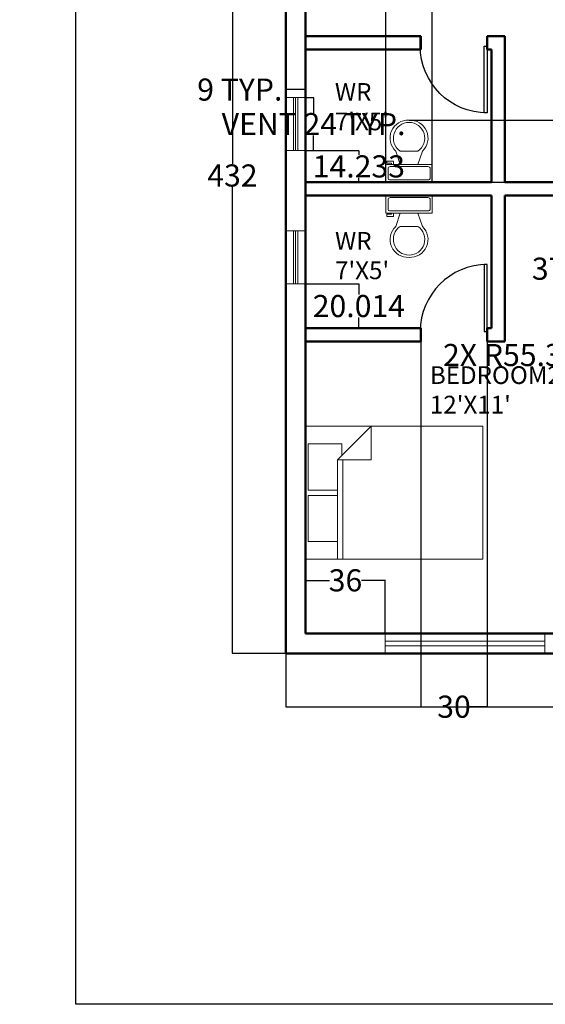
# Model space of a CAD drawing. Units: inches. Extents: x -16 to 1298, y 3 to 744.
# Tile 1 of 5: x -16 to 221, y 3 to 448. Entities that reach past the tile are written whole.
import ezdxf

# ---------------------------------------------------------------- set-up
doc = ezdxf.new("R2010")
doc.units = ezdxf.units.IN
doc.header["$MEASUREMENT"] = 0
for name, color, linetype, lineweight in [('A-ANNO-DIMS', 2, 'Continuous', 18), ('A-AREA-IDEN', 7, 'Continuous', 18), ('A-DOOR', 3, 'Continuous', 25), ('A-FLOR-FIXT', 9, 'Continuous', 18), ('A-FURN', 8, 'Continuous', 18), ('A-GLAZ', 4, 'Continuous', 18), ('A-WALL', 7, 'Continuous', 50)]:
    doc.layers.add(name, color=color, linetype=linetype, lineweight=lineweight)
doc.styles.get("Standard").update_dxf_attribs({"font": 'arial.ttf'})
doc.dimstyles.get("Standard").update_dxf_attribs({"dimtxt": 10, "dimasz": 0.18, "dimexe": 0.18, "dimexo": 0.0625, "dimgap": 0.09, "dimtad": 0, "dimtih": 1, "dimtoh": 1, "dimdec": 0, "dimzin": 0, "dimdsep": 46, "dimlunit": 3, "dimtxsty": 'Standard', "dimcen": 0.09, "dimadec": 0, "dimazin": 0, "dimtfac": 1, "dimtdec": 0, "dimtofl": 0, "dimtmove": 0, "dimatfit": 3, "dimfxl": 1, "dimtolj": 1, "dimtzin": 0, "dimarcsym": 0})

# ---------------------------------------------------------------- blocks, each defined once
blk = doc.blocks.new('Bed - Queen')
for p, q in [((0, -80.00003), (0, 0)), ((0, 0), (59.99999, 0)), ((59.99999, 0), (59.99999, -80.00003)), ((7.99999, -1.2), (28.79998, -1.2)), ((7.99999, -14.4), (7.99999, -1.2)), ((28.79998, -1.2), (28.79998, -14.4)), ((31.19999, -1.2), (51.99999, -1.2)), ((31.19999, -14.4), (31.19999, -1.2)), ((51.99999, -1.2), (51.99999, -16.4)), ((0, -14.4), (44.8, -14.4)), ((44.8, -16.8), (0, -16.8)), ((59.99999, -29.6), (44.8, -14.4)), ((44.8, -14.4), (44.8, -29.6)), ((51.99999, -16.4), (46.79936, -16.4)), ((44.8, -29.6), (59.99999, -29.6)), ((59.99999, -80.00003), (0, -80.00003))]:
    blk.add_line(p, q)
blk = doc.blocks.new('*U8')
for p, q in [((0, 0), (0, -6)), ((-40, 0), (-40, -6))]:
    blk.add_line(p, q)
blk.add_lwpolyline([(0, 0), (0, 40), (-1.75, 40), (-1.75, 0)], close=True)
blk.add_arc((0, 0), 40, 90, 180)
blk = doc.blocks.new('*U3')
for p, q in [((9.5, -6), (9.5, -2)), ((-10, -8.5), (-8, -8.5)), ((-10, -9.5), (-10, -8.5)), ((-8, -8.5), (-8, -8)), ((-7, -8), (-7, -9.5)), ((-4, -8), (-6, -14)), ((4, -8), (6, -14)), ((-7, -9.5), (-10, -9.5)), ((4, -14), (-4, -14))]:
    blk.add_line(p, q)
blk.add_lwpolyline([(10.5, -8), (10.5, 0), (-10.5, 0), (-10.5, -8)], close=True)
for points in [[(-9.5, -2), (-9.5, -6)], [(8.5, -1), (-8.5, -1)], [(-8.5, -7), (8.5, -7)]]:
    blk.add_lwpolyline(points)
for centre, radius, start, end in [((-8.625, -1.875), 0.8839, 81.8699, 188.1301), ((8.625, -1.875), 0.8839, 351.8699, 98.1301), ((-8.625, -6.125), 0.8839, 171.869898, 278.1301), ((8.625, -6.125), 0.8839, 261.8699, 8.1301), ((-0.4772, -19.9188), 8.0953, 133.01722, 273.38), ((0.0374, -19.8731), 7.127, 124.50543, 269.7), ((-0.0373, -19.8731), 7.127, 270.3, 55.4946), ((0.4773, -19.9188), 8.0953, 266.62, 46.9828)]:
    blk.add_arc(centre, radius, start, end)
blk = doc.blocks.new('WIN-72-WALL-9')
for p, q in [((0, 0), (0, 9)), ((72, 0), (72, 9)), ((72, 5.5), (0, 5.5)), ((72, 3.5), (0, 3.5))]:
    blk.add_line(p, q)
blk = doc.blocks.new('VENT-24-WALL-9')
for p, q in [((0, 0), (0, 9)), ((24, 0), (24, 9)), ((0, 5.5), (24, 5.5)), ((0, 4.5), (24, 4.5)), ((0, 3.5), (24, 3.5))]:
    blk.add_line(p, q)
blk = doc.blocks.new('*D28')
at = {"layer": 'A-ANNO-DIMS', "color": 0, "lineweight": -2, "transparency": 16777216}
for p, q in [((112.74, 413.22), (116.46, 413.22)), ((116.28, 413.04), (116.28, 406.34)), ((116.28, 389.4), (116.28, 396.11)), ((112.74, 389.22), (116.46, 389.22))]:
    blk.add_line(p, q, dxfattribs=at)
at = {"layer": 'A-ANNO-DIMS', "color": 0, "transparency": 16777216}
for points in [[(116.25, 413.04), (116.31, 413.04), (116.28, 413.22)], [(116.25, 389.4), (116.31, 389.4), (116.28, 389.22)]]:
    blk.add_solid(points, dxfattribs=at)
at = {"layer": 'Defpoints', "color": 0, "transparency": 16777216}
for p in [(112.68, 413.22), (116.28, 413.22), (112.68, 389.22)]:
    blk.add_point(p, dxfattribs=at)
at = {"layer": 'A-ANNO-DIMS', "color": 0, "transparency": 16777216, "insert": (116.28, 401.22), "char_height": 10, "attachment_point": 5}
blk.add_mtext('\\A1;VENT 24 TYP.', dxfattribs=at)
blk = doc.blocks.new('*D29')
at = {"layer": 'A-ANNO-DIMS', "color": 0, "lineweight": -2, "transparency": 16777216}
for p, q in [((103.68, 416.82), (103.5, 416.82)), ((103.68, 413.28), (103.68, 417)), ((112.5, 416.82), (103.86, 416.82)), ((112.68, 413.28), (112.68, 417))]:
    blk.add_line(p, q, dxfattribs=at)
at = {"layer": 'A-ANNO-DIMS', "color": 0, "transparency": 16777216}
for points in [[(103.86, 416.85), (103.86, 416.79), (103.68, 416.82)], [(112.5, 416.85), (112.5, 416.79), (112.68, 416.82)]]:
    blk.add_solid(points, dxfattribs=at)
at = {"layer": 'Defpoints', "color": 0, "transparency": 16777216}
for p in [(103.68, 416.82), (103.68, 413.22), (112.68, 413.22)]:
    blk.add_point(p, dxfattribs=at)
at = {"layer": 'A-ANNO-DIMS', "color": 0, "transparency": 16777216, "insert": (82.95, 416.82), "char_height": 10, "attachment_point": 5}
blk.add_mtext('\\A1;9 TYP.', dxfattribs=at)
blk = doc.blocks.new('*D30')
at = {"layer": 'A-ANNO-DIMS', "color": 0, "lineweight": -2, "transparency": 16777216}
for p, q in [((112.68, 484.49), (112.68, 472.37)), ((192.68, 484.49), (192.68, 472.37)), ((112.68, 472.55), (112.5, 472.55)), ((192.5, 472.55), (112.86, 472.55))]:
    blk.add_line(p, q, dxfattribs=at)
at = {"layer": 'A-ANNO-DIMS', "color": 0, "transparency": 16777216}
for points in [[(112.86, 472.58), (112.86, 472.52), (112.68, 472.55)], [(192.5, 472.58), (192.5, 472.52), (192.68, 472.55)]]:
    blk.add_solid(points, dxfattribs=at)
at = {"layer": 'Defpoints', "color": 0, "transparency": 16777216}
for p in [(112.68, 484.55), (192.68, 484.55), (112.68, 472.55)]:
    blk.add_point(p, dxfattribs=at)
at = {"layer": 'A-ANNO-DIMS', "color": 0, "transparency": 16777216, "insert": (45, 472.55), "char_height": 10, "attachment_point": 5}
blk.add_mtext('\\A1;QUEEN BED 80 TYP.', dxfattribs=at)
blk = doc.blocks.new('*D33')
at = {"layer": 'A-ANNO-DIMS', "color": 0, "lineweight": -2, "transparency": 16777216}
for p, q in [((262.47, 335.87), (262.29, 335.87)), ((262.47, 326.93), (262.47, 336.05)), ((298.96, 335.87), (262.65, 335.87)), ((299.14, 326.93), (299.14, 336.05))]:
    blk.add_line(p, q, dxfattribs=at)
at = {"layer": 'A-ANNO-DIMS', "color": 0, "transparency": 16777216}
for points in [[(262.65, 335.9), (262.65, 335.84), (262.47, 335.87)], [(298.96, 335.9), (298.96, 335.84), (299.14, 335.87)]]:
    blk.add_solid(points, dxfattribs=at)
at = {"layer": 'Defpoints', "color": 0, "transparency": 16777216}
for p in [(262.47, 335.87), (262.47, 326.87), (299.14, 326.87)]:
    blk.add_point(p, dxfattribs=at)
at = {"layer": 'A-ANNO-DIMS', "color": 0, "transparency": 16777216, "insert": (237.87, 335.87), "char_height": 10, "attachment_point": 5}
blk.add_mtext('\\A1;37 TYP.', dxfattribs=at)
blk = doc.blocks.new('*D40')
at = {"layer": 'A-ANNO-DIMS', "color": 0, "lineweight": -2, "transparency": 16777216}
for p, q in [((103.68, 161.93), (103.68, 137.76)), ((487.68, 161.93), (487.68, 137.76)), ((103.86, 137.94), (284.56, 137.94)), ((487.5, 137.94), (306.79, 137.94))]:
    blk.add_line(p, q, dxfattribs=at)
at = {"layer": 'A-ANNO-DIMS', "color": 0, "transparency": 16777216}
for points in [[(103.86, 137.97), (103.86, 137.91), (103.68, 137.94)], [(487.5, 137.97), (487.5, 137.91), (487.68, 137.94)]]:
    blk.add_solid(points, dxfattribs=at)
at = {"layer": 'Defpoints', "color": 0, "transparency": 16777216}
for p in [(103.68, 161.99), (487.68, 161.99), (487.68, 137.94)]:
    blk.add_point(p, dxfattribs=at)
at = {"layer": 'A-ANNO-DIMS', "color": 0, "transparency": 16777216, "insert": (295.68, 137.94), "char_height": 10, "attachment_point": 5}
blk.add_mtext('\\A1;384', dxfattribs=at)
blk = doc.blocks.new('*D41')
at = {"layer": 'A-ANNO-DIMS', "color": 0, "lineweight": -2, "transparency": 16777216}
for p, q in [((103.61, 593.99), (79.45, 593.99)), ((79.63, 593.81), (79.63, 383.19)), ((79.63, 162.17), (79.63, 372.79)), ((103.61, 161.99), (79.45, 161.99))]:
    blk.add_line(p, q, dxfattribs=at)
at = {"layer": 'A-ANNO-DIMS', "color": 0, "transparency": 16777216}
for points in [[(79.6, 593.81), (79.66, 593.81), (79.63, 593.99)], [(79.6, 162.17), (79.66, 162.17), (79.63, 161.99)]]:
    blk.add_solid(points, dxfattribs=at)
at = {"layer": 'Defpoints', "color": 0, "transparency": 16777216}
for p in [(79.63, 593.99), (103.68, 593.99), (103.68, 161.99)]:
    blk.add_point(p, dxfattribs=at)
at = {"layer": 'A-ANNO-DIMS', "color": 0, "transparency": 16777216, "insert": (79.63, 377.99), "char_height": 10, "attachment_point": 5}
blk.add_mtext('\\A1;432', dxfattribs=at)
blk = doc.blocks.new('*D48')
at = {"layer": 'A-ANNO-DIMS', "color": 0, "lineweight": -2, "transparency": 16777216}
for p, q in [((112.68, 171.05), (112.68, 195.22)), ((112.86, 195.04), (123.43, 195.04)), ((148.5, 195.04), (137.92, 195.04)), ((148.68, 171.05), (148.68, 195.22))]:
    blk.add_line(p, q, dxfattribs=at)
at = {"layer": 'A-ANNO-DIMS', "color": 0, "transparency": 16777216}
for points in [[(112.86, 195.07), (112.86, 195.01), (112.68, 195.04)], [(148.5, 195.07), (148.5, 195.01), (148.68, 195.04)]]:
    blk.add_solid(points, dxfattribs=at)
at = {"layer": 'Defpoints', "color": 0, "transparency": 16777216}
for p in [(148.68, 195.04), (112.68, 170.99), (148.68, 170.99)]:
    blk.add_point(p, dxfattribs=at)
at = {"layer": 'A-ANNO-DIMS', "color": 0, "transparency": 16777216, "insert": (130.68, 195.04), "char_height": 10, "attachment_point": 5}
blk.add_mtext('\\A1;36', dxfattribs=at)
blk = doc.blocks.new('*D53')
at = {"layer": 'A-ANNO-DIMS', "color": 0, "lineweight": -2, "transparency": 16777216}
for p, q in [((164.68, 302.93), (164.68, 137.76)), ((194.68, 302.93), (194.68, 137.76)), ((164.86, 137.94), (172.44, 137.94)), ((194.5, 137.94), (186.91, 137.94))]:
    blk.add_line(p, q, dxfattribs=at)
at = {"layer": 'A-ANNO-DIMS', "color": 0, "transparency": 16777216}
for points in [[(164.86, 137.97), (164.86, 137.91), (164.68, 137.94)], [(194.5, 137.97), (194.5, 137.91), (194.68, 137.94)]]:
    blk.add_solid(points, dxfattribs=at)
at = {"layer": 'Defpoints', "color": 0, "transparency": 16777216}
for p in [(164.68, 302.99), (194.68, 302.99), (194.68, 137.94)]:
    blk.add_point(p, dxfattribs=at)
at = {"layer": 'A-ANNO-DIMS', "color": 0, "transparency": 16777216, "insert": (179.68, 137.94), "char_height": 10, "attachment_point": 5}
blk.add_mtext('\\A1;30', dxfattribs=at)
blk = doc.blocks.new('*D59')
at = {"layer": 'A-ANNO-DIMS', "color": 0, "lineweight": -2, "transparency": 16777216}
for p, q in [((112.74, 389.22), (136.91, 389.22)), ((136.73, 389.04), (136.73, 387.3)), ((112.74, 374.99), (136.91, 374.99)), ((136.73, 375.17), (136.73, 376.91))]:
    blk.add_line(p, q, dxfattribs=at)
at = {"layer": 'A-ANNO-DIMS', "color": 0, "transparency": 16777216}
for points in [[(136.7, 389.04), (136.76, 389.04), (136.73, 389.22)], [(136.7, 375.17), (136.76, 375.17), (136.73, 374.99)]]:
    blk.add_solid(points, dxfattribs=at)
at = {"layer": 'Defpoints', "color": 0, "transparency": 16777216}
for p in [(112.68, 389.22), (112.68, 374.99), (136.73, 374.99)]:
    blk.add_point(p, dxfattribs=at)
at = {"layer": 'A-ANNO-DIMS', "color": 0, "transparency": 16777216, "insert": (136.73, 382.1), "char_height": 10, "attachment_point": 5}
blk.add_mtext('\\A1;14.233', dxfattribs=at)
blk = doc.blocks.new('*D60')
at = {"layer": 'A-ANNO-DIMS', "color": 0, "lineweight": -2, "transparency": 16777216}
for p, q in [((112.74, 329), (136.91, 329)), ((136.73, 328.82), (136.73, 324.19)), ((136.73, 309.17), (136.73, 313.8)), ((112.74, 308.99), (136.91, 308.99))]:
    blk.add_line(p, q, dxfattribs=at)
at = {"layer": 'A-ANNO-DIMS', "color": 0, "transparency": 16777216}
for points in [[(136.7, 328.82), (136.76, 328.82), (136.73, 329)], [(136.7, 309.17), (136.76, 309.17), (136.73, 308.99)]]:
    blk.add_solid(points, dxfattribs=at)
at = {"layer": 'Defpoints', "color": 0, "transparency": 16777216}
for p in [(112.68, 329), (112.68, 308.99), (136.73, 308.99)]:
    blk.add_point(p, dxfattribs=at)
at = {"layer": 'A-ANNO-DIMS', "color": 0, "transparency": 16777216, "insert": (136.73, 319), "char_height": 10, "attachment_point": 5}
blk.add_mtext('\\A1;20.014', dxfattribs=at)
blk = doc.blocks.new('*D61')
at = {"layer": 'A-ANNO-DIMS', "color": 0, "lineweight": -2, "transparency": 16777216}
for p, q in [((148.9, 375.05), (148.9, 618.22)), ((149.08, 618.04), (153.03, 618.04)), ((169.72, 618.04), (165.77, 618.04)), ((169.9, 375.05), (169.9, 618.22))]:
    blk.add_line(p, q, dxfattribs=at)
at = {"layer": 'A-ANNO-DIMS', "color": 0, "transparency": 16777216}
for points in [[(149.08, 618.07), (149.08, 618.01), (148.9, 618.04)], [(169.72, 618.07), (169.72, 618.01), (169.9, 618.04)]]:
    blk.add_solid(points, dxfattribs=at)
at = {"layer": 'Defpoints', "color": 0, "transparency": 16777216}
for p in [(169.9, 618.04), (148.9, 374.99), (169.9, 374.99)]:
    blk.add_point(p, dxfattribs=at)
at = {"layer": 'A-ANNO-DIMS', "color": 0, "transparency": 16777216, "insert": (159.4, 618.04), "char_height": 10, "attachment_point": 5}
blk.add_mtext('\\A1;21', dxfattribs=at)
blk = doc.blocks.new('*D62')
at = {"layer": 'A-ANNO-DIMS', "color": 0, "lineweight": -2, "transparency": 16777216}
for p, q in [((159.46, 402.99), (511.91, 402.99)), ((511.73, 402.81), (511.73, 394.18)), ((511.73, 375.17), (511.73, 383.79)), ((169.96, 374.99), (511.91, 374.99))]:
    blk.add_line(p, q, dxfattribs=at)
at = {"layer": 'A-ANNO-DIMS', "color": 0, "transparency": 16777216}
for points in [[(511.7, 402.81), (511.76, 402.81), (511.73, 402.99)], [(511.7, 375.17), (511.76, 375.17), (511.73, 374.99)]]:
    blk.add_solid(points, dxfattribs=at)
at = {"layer": 'Defpoints', "color": 0, "transparency": 16777216}
for p in [(159.4, 402.99), (511.73, 402.99), (169.9, 374.99)]:
    blk.add_point(p, dxfattribs=at)
at = {"layer": 'A-ANNO-DIMS', "color": 0, "transparency": 16777216, "insert": (511.73, 388.99), "char_height": 10, "attachment_point": 5}
blk.add_mtext('\\A1;28', dxfattribs=at)
blk = doc.blocks.new('*D88')
at = {"layer": 'A-ANNO-DIMS', "color": 0, "lineweight": -2, "transparency": 16777216}
for p, q in [((237.91, 296.87), (270.96, 296.87)), ((326.43, 296.87), (326.61, 296.87)), ((326.52, 296.78), (326.52, 296.96))]:
    blk.add_line(p, q, dxfattribs=at)
at = {"layer": 'A-ANNO-DIMS', "color": 0, "transparency": 16777216}
blk.add_solid([(270.96, 296.9), (270.96, 296.84), (271.14, 296.87)], dxfattribs=at)
at = {"layer": 'Defpoints', "color": 0, "transparency": 16777216}
for p in [(271.14, 296.87), (326.52, 296.87)]:
    blk.add_point(p, dxfattribs=at)
at = {"layer": 'A-ANNO-DIMS', "color": 0, "transparency": 16777216, "insert": (205.32, 296.87), "char_height": 10, "attachment_point": 5}
blk.add_mtext('\\A1;2X R55.38', dxfattribs=at)

msp = doc.modelspace()

# ---------------------------------------------------------------- linework, layer by layer
at = {"layer": 'A-WALL'}
for p, q in [((103.6768, 593.9884), (103.6768, 161.9884)), ((112.6768, 584.9884), (112.6768, 170.9884)), ((164.6768, 440.9884), (112.6768, 440.9884)), ((164.6768, 440.9884), (164.6768, 434.9884)), ((196.6768, 440.9884), (194.6768, 440.9884)), ((194.6768, 440.9884), (194.6768, 434.9884)), ((202.6768, 440.9884), (196.6768, 440.9884)), ((202.6768, 440.9884), (202.6768, 374.9884)), ((164.6768, 434.9884), (112.6768, 434.9884)), ((194.6768, 434.9884), (196.6768, 434.9884)), ((196.6768, 434.9884), (196.6768, 374.9884)), ((196.6768, 374.9884), (112.6768, 374.9884)), ((256.6768, 374.9884), (202.6768, 374.9884)), ((196.6768, 368.9884), (112.6768, 368.9884)), ((196.6768, 368.9884), (196.6768, 308.9884)), ((256.6768, 368.9884), (202.6768, 368.9884)), ((202.6768, 368.9884), (202.6768, 302.9884)), ((164.6768, 308.9884), (112.6768, 308.9884)), ((164.6768, 308.9884), (164.6768, 302.9884)), ((194.6768, 302.9884), (194.6768, 308.9884)), ((194.6768, 308.9884), (196.6768, 308.9884)), ((164.6768, 302.9884), (112.6768, 302.9884)), ((196.6768, 302.9884), (194.6768, 302.9884)), ((202.6768, 302.9884), (196.6768, 302.9884)), ((112.6768, 170.9884), (262.6768, 170.9884)), ((112.6768, 170.9884), (256.6768, 170.9884)), ((103.6768, 161.9884), (487.6768, 161.9884))]:
    msp.add_line(p, q, dxfattribs=at)
at = {"layer": 'Defpoints'}
msp.add_lwpolyline([(8.9336, 744.17), (1298.346, 744.17), (1298.346, 3.4476), (8.9336, 3.4476)], close=True, dxfattribs=at)

# ---------------------------------------------------------------- block references
at = {"layer": 'A-DOOR', "xscale": -0.7552380589311617, "yscale": 0.7552380589311617, "zscale": 0.7552380589311617, "rotation": 180}
msp.add_blockref('*U8', (194.6768, 436.4569), dxfattribs=at)
at = {"layer": 'A-DOOR', "xscale": 0.7552380589311617, "yscale": 0.7552380589311617, "zscale": 0.7552380589311617}
msp.add_blockref('*U8', (194.6768, 307.5198), dxfattribs=at)
at = {"layer": 'A-FLOR-FIXT', "xscale": -1, "rotation": 180}
msp.add_blockref('*U3', (159.3975, 374.9884), dxfattribs=at)
at = {"layer": 'A-FLOR-FIXT'}
msp.add_blockref('*U3', (159.3975, 368.9884), dxfattribs=at)
at = {"layer": 'A-FURN', "rotation": 90}
msp.add_blockref('Bed - Queen', (112.6768, 204.6521), dxfattribs=at)
at = {"layer": 'A-GLAZ'}
for name, p, rotation in [('VENT-24-WALL-9', (112.6768, 389.2212), 90.00000000000067), ('VENT-24-WALL-9', (112.6768, 329.0025), 90.00000000000067), ('WIN-72-WALL-9', (220.6768, 170.9884), 180)]:
    msp.add_blockref(name, p, dxfattribs=dict(at, rotation=rotation))

# ---------------------------------------------------------------- texts
at = {"layer": 'A-AREA-IDEN', "char_height": 8, "attachment_point": 1}
for s, insert in [("WR\\P7'X5'", (125.9004, 419.7607)), ("WR\\P7'X5'", (125.967, 352.4654)), ("BEDROOM2\\P12'X11'", (168.8016, 291.7695))]:
    msp.add_mtext_dynamic_manual_height_columns(s, width=63.245227, gutter_width=1, heights=[0], dxfattribs=dict(at, insert=insert))

# ---------------------------------------------------------------- dimensions: what is measured, and where the dimension line sits
at = {"layer": 'A-ANNO-DIMS'}
for base, p1, p2, picture, middle in [((169.8975, 618.0384), (148.8975, 374.9884), (169.8975, 374.9884), '*D61', (159.3975, 618.0384)), ((194.6768, 137.9384), (164.6768, 302.9884), (194.6768, 302.9884), '*D53', (179.6768, 137.9384)), ((148.6768, 195.0384), (112.6768, 170.9884), (148.6768, 170.9884), '*D48', (130.6768, 195.0384)), ((487.6768, 137.9384), (103.6768, 161.9884), (487.6768, 161.9884), '*D40', (295.6768, 137.9384))]:
    dim = msp.add_linear_dim(base=base, p1=p1, p2=p2, dimstyle='Standard', override={"dimdec": 0, "dimlfac": 1, "dimrnd": 0, "dimzin": 0, "dimdsep": 46, "dimlunit": 2}, dxfattribs=at)
    dim.commit()
    dim.dimension.update_dxf_attribs({"geometry": picture, "text_midpoint": middle})
for base, p1, p2, angle, override, picture, middle in [((79.6268, 593.9884), (103.6768, 161.9884), (103.6768, 593.9884), 90, {"dimdec": 0, "dimlfac": 1, "dimrnd": 0, "dimzin": 0, "dimdsep": 46, "dimlunit": 2}, '*D41', (79.6268, 377.9884)), ((511.7268, 402.9883), (169.8975, 374.9884), (159.3976, 402.9883), 90, {"dimdec": 0, "dimlfac": 1, "dimrnd": 0, "dimzin": 0, "dimdsep": 46, "dimlunit": 2}, '*D62', (511.7268, 388.9884)), ((136.7268, 374.9884), (112.6768, 389.2212), (112.6768, 374.9884), 270, {"dimdec": 3, "dimlfac": 1, "dimrnd": 0, "dimzin": 0, "dimdsep": 46, "dimlunit": 2}, '*D59', (136.7268, 382.1048)), ((136.7268, 308.9884), (112.6768, 329.0025), (112.6768, 308.9884), 270, {"dimdec": 3, "dimlfac": 1, "dimrnd": 0, "dimzin": 0, "dimdsep": 46, "dimlunit": 2}, '*D60', (136.7268, 318.9954))]:
    dim = msp.add_linear_dim(base=base, p1=p1, p2=p2, angle=angle, dimstyle='Standard', override=override, dxfattribs=at)
    dim.commit()
    dim.dimension.update_dxf_attribs({"geometry": picture, "text_midpoint": middle})
for base, p1, p2, angle, text, picture, middle in [((112.6768, 472.5483), (192.6768, 484.5483), (112.6768, 484.5483), 180, 'QUEEN BED <> TYP.', '*D30', (44.9955, 472.5483)), ((103.6768, 416.8212), (112.6768, 413.2212), (103.6768, 413.2212), 180, '<> TYP.', '*D29', (82.9532, 416.8212)), ((116.2768, 413.2212), (112.6768, 389.2212), (112.6768, 413.2212), 90, 'VENT <> TYP.', '*D28', (116.2768, 401.2212)), ((262.4712, 335.8707), (299.1378, 326.8707), (262.4712, 326.8707), 180, '<> TYP.', '*D33', (237.8662, 335.8707))]:
    dim = msp.add_linear_dim(base=base, p1=p1, p2=p2, angle=angle, text=text, dimstyle='Standard', override={"dimdec": 0, "dimlfac": 1, "dimrnd": 0, "dimzin": 0, "dimdsep": 46, "dimlunit": 2}, dxfattribs=at)
    dim.commit()
    dim.dimension.update_dxf_attribs({"geometry": picture, "text_midpoint": middle})
dim = msp.add_radius_dim(center=(326.5222, 296.8707), mpoint=(271.1378, 296.871), text='2X <>', dimstyle='Standard', override={"dimdec": 2, "dimlfac": 1, "dimrnd": 0, "dimzin": 0, "dimdsep": 46, "dimlunit": 2}, dxfattribs=at)
dim.commit()
dim.dimension.update_dxf_attribs({"geometry": '*D88', "text_midpoint": (237.9071, 296.8712), "dimtype": 164})

doc.saveas('drawing.dxf')
